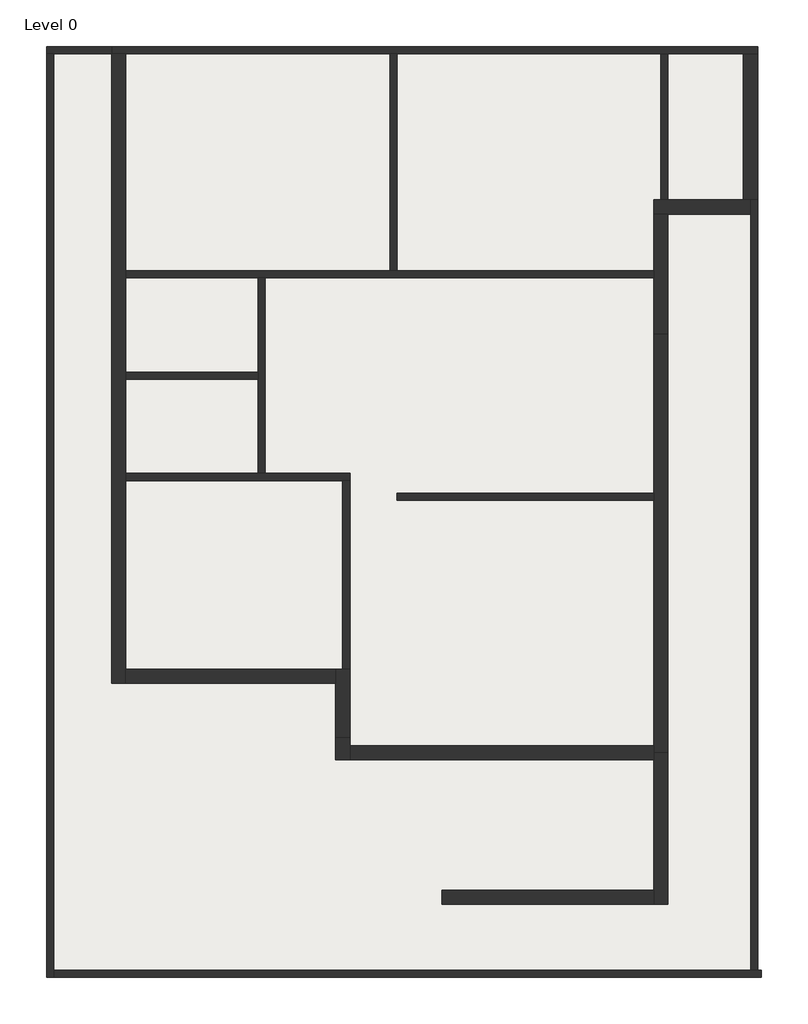
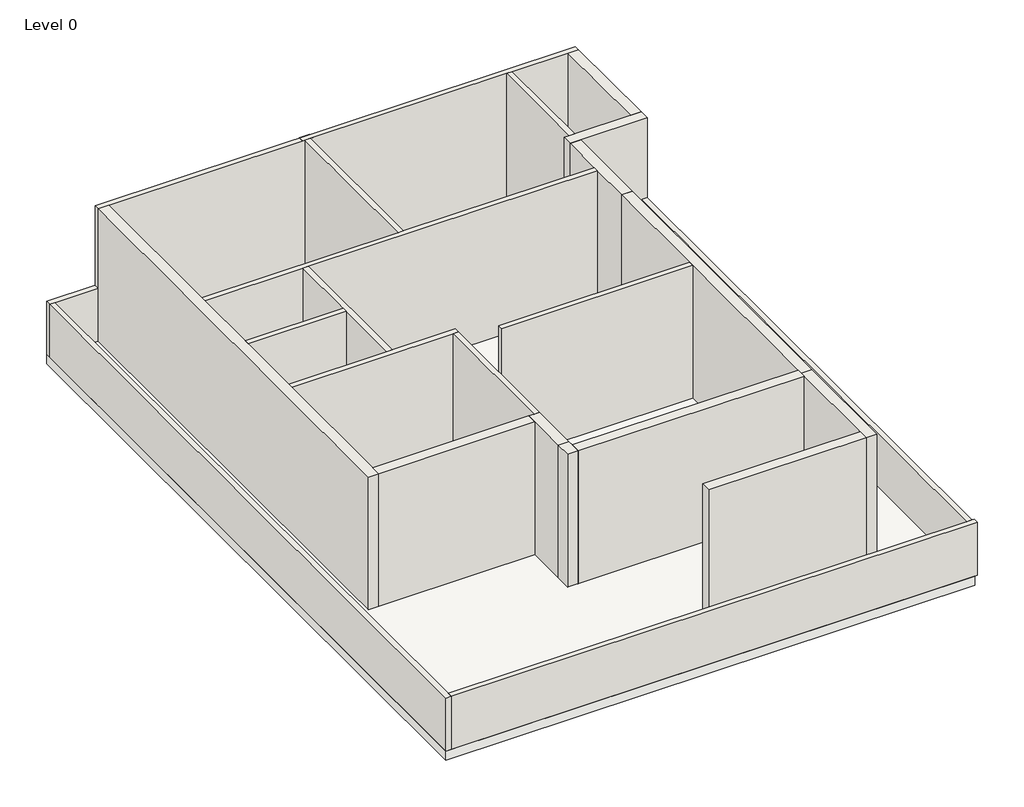
# One storey: 25 walls, 1 slab.
"""IFC4 building model written with IfcOpenShell, lengths in millimetres."""

from ifc_helpers import new_model, si_unit, frame, origin, origin_with_axes, place, context, project, spatial, polyline, outline, extrude, faceted_brep, element, save

model = new_model("IFC4")

# Units and contexts
model_context = context("Model", 3, world=origin())
ifc_project = project(units=[si_unit("LENGTHUNIT", "METRE", prefix="MILLI")], contexts=[model_context])

# Site, building, storey
site = spatial("IfcSite", under=ifc_project)
building = spatial("IfcBuilding", under=site)
storey = spatial("IfcBuildingStorey", under=building, Name="Level 0", Elevation=0.0)

# Slab
placement = place(None, origin())
element("IfcSlab", 1, at=placement, inside=storey, context=model_context, shape_type="SweptSolid", body=[
    extrude(outline(polyline([(5920.3326329, 7268.7468257), (5920.3326329, -7768.0531743), (-5573.1673671, -7768.0531743), (-5573.1673671, 7268.7468257), (5920.3326329, 7268.7468257)])), frame((0.0, 0.0, -211.0), z_axis=(0.0, 0.0, 1.0), x_axis=(1.0, 0.0, 0.0)), (0.0, 0.0, 1.0), 211.0),
])

# Walls
element("IfcWall", 2, ObjectType="INNER WALL-4.5\"", at=placement, inside=storey, context=model_context, shape_type="Brep", body=[
    faceted_brep([(-5573.1673671, 7154.4468257, 0.0), (-5458.8673671, 7154.4468257, 0.0), (-4519.0673671, 7154.4468257, 0.0), (-4519.0673671, 7154.4468257, 1219.2), (-5458.8673671, 7154.4468257, 1219.2), (-5573.1673671, 7154.4468257, 1219.2), (-5573.1673671, 7268.7468257, 0.0), (-5573.1673671, 7268.7468257, 1219.2), (-4519.0673671, 7268.7468257, 1219.2), (-4519.0673671, 7268.7468257, 0.0)], [[[0, 1, 2, 3, 4, 5]], [[6, 7, 8, 9]], [[2, 1, 0, 6, 9]], [[3, 2, 9, 8]], [[5, 4, 3, 8, 7]], [[0, 5, 7, 6]]]),
])
element("IfcWall", 3, ObjectType="INNER WALL-4.5\"", at=placement, inside=storey, context=model_context, shape_type="Brep", body=[
    faceted_brep([(-5573.1673671, 7154.4468257, 0.0), (-5573.1673671, -7768.0531743, 0.0), (-5573.1673671, -7768.0531743, 1219.2), (-5573.1673671, 7154.4468257, 1219.2), (-5458.8673671, 7154.4468257, 0.0), (-5458.8673671, 7154.4468257, 1219.2), (-5458.8673671, -7653.7531743, 1219.2), (-5458.8673671, -7768.0531743, 1219.2), (-5458.8673671, -7768.0531743, 0.0), (-5458.8673671, -7653.7531743, 0.0)], [[[0, 1, 2, 3]], [[4, 5, 6, 7, 8, 9]], [[1, 0, 4, 9, 8]], [[3, 2, 7, 6, 5]], [[0, 3, 5, 4]], [[2, 1, 8, 7]]]),
])
element("IfcWall", 4, ObjectType="INNER WALL-4.5\"", at=placement, inside=storey, context=model_context, shape_type="Brep", body=[
    faceted_brep([(5977.4826329, -7653.7531743, 0.0), (5920.3326329, -7653.7531743, 0.0), (5806.0326329, -7653.7531743, 0.0), (-5458.8673671, -7653.7531743, 0.0), (-5458.8673671, -7653.7531743, 1219.2), (5806.0326329, -7653.7531743, 1219.2), (5920.3326329, -7653.7531743, 1219.2), (5977.4826329, -7653.7531743, 1219.2), (5977.4826329, -7768.0531743, 0.0), (5977.4826329, -7768.0531743, 1219.2), (-5458.8673671, -7768.0531743, 1219.2), (-5458.8673671, -7768.0531743, 0.0)], [[[0, 1, 2, 3, 4, 5, 6, 7]], [[8, 9, 10, 11]], [[3, 2, 1, 0, 8, 11]], [[7, 6, 5, 4, 10, 9]], [[0, 7, 9, 8]], [[4, 3, 11, 10]]]),
])
element("IfcWall", 5, ObjectType="INNER WALL-4.5\"", at=placement, inside=storey, context=model_context, shape_type="Brep", body=[
    faceted_brep([(5806.0326329, 4792.2468257, 0.0), (5806.0326329, 4563.6468257, 0.0), (5806.0326329, -7653.7531743, 0.0), (5806.0326329, -7653.7531743, 1219.2), (5806.0326329, 4563.6468257, 1219.2), (5806.0326329, 4792.2468257, 1219.2), (5920.3326329, 4792.2468257, 0.0), (5920.3326329, 4792.2468257, 1219.2), (5920.3326329, 4563.6468257, 1219.2), (5920.3326329, -7653.7531743, 1219.2), (5920.3326329, -7653.7531743, 0.0)], [[[0, 1, 2, 3, 4, 5]], [[6, 7, 8, 9, 10]], [[2, 1, 0, 6, 10]], [[5, 4, 3, 9, 8, 7]], [[3, 2, 10, 9]], [[0, 5, 7, 6]]]),
])
element("IfcWall", 6, ObjectType="INNER WALL-4.5\"", at=placement, inside=storey, context=model_context, shape_type="Brep", body=[
    faceted_brep([(-4519.0673671, 7154.4468257, 0.0), (-4290.4673671, 7154.4468257, 0.0), (-23.2673671, 7154.4468257, 0.0), (91.0326329, 7154.4468257, 0.0), (4358.2326329, 7154.4468257, 0.0), (4472.5326329, 7154.4468257, 0.0), (5691.7326329, 7154.4468257, 0.0), (5920.3326329, 7154.4468257, 0.0), (5920.3326329, 7154.4468257, 3048.0), (5691.7326329, 7154.4468257, 3048.0), (4472.5326329, 7154.4468257, 3048.0), (4358.2326329, 7154.4468257, 3048.0), (91.0326329, 7154.4468257, 3048.0), (-23.2673671, 7154.4468257, 3048.0), (-4290.4673671, 7154.4468257, 3048.0), (-4519.0673671, 7154.4468257, 3048.0), (-4519.0673671, 7154.4468257, 1219.2), (-4519.0673671, 7268.7468257, 0.0), (-4519.0673671, 7268.7468257, 1219.2), (-4519.0673671, 7268.7468257, 3048.0), (5920.3326329, 7268.7468257, 3048.0), (5920.3326329, 7268.7468257, 0.0)], [[[0, 1, 2, 3, 4, 5, 6, 7, 8, 9, 10, 11, 12, 13, 14, 15, 16]], [[17, 18, 19, 20, 21]], [[7, 6, 5, 4, 3, 2, 1, 0, 17, 21]], [[15, 14, 13, 12, 11, 10, 9, 8, 20, 19]], [[0, 16, 15, 19, 18, 17]], [[8, 7, 21, 20]]]),
])
element("IfcWall", 7, ObjectType="INNER WALL-4.5\"", at=placement, inside=storey, context=model_context, shape_type="Brep", body=[
    faceted_brep([(148.1826329, 7268.7468257, 0.0), (-80.4173671, 7268.7468257, 0.0), (-80.4173671, 7268.7468257, 3048.0), (148.1826329, 7268.7468257, 3048.0), (148.1826329, 7154.4468257, 0.0), (148.1826329, 7154.4468257, 3048.0), (91.0326329, 7154.4468257, 3048.0), (-23.2673671, 7154.4468257, 3048.0), (-80.4173671, 7154.4468257, 3048.0), (-80.4173671, 7154.4468257, 0.0), (-23.2673671, 7154.4468257, 0.0), (91.0326329, 7154.4468257, 0.0)], [[[0, 1, 2, 3]], [[4, 5, 6, 7, 8, 9, 10, 11]], [[1, 0, 4, 11, 10, 9]], [[2, 1, 9, 8]], [[3, 2, 8, 7, 6, 5]], [[0, 3, 5, 4]]]),
])
element("IfcWall", 8, ObjectType="INNER WALL-4.5\"", at=placement, inside=storey, context=model_context, shape_type="SweptSolid", body=[
    extrude(outline(polyline([(-23.2673671, 3649.2468257), (-23.2673671, 7154.4468257), (91.0326329, 7154.4468257), (91.0326329, 3649.2468257), (-23.2673671, 3649.2468257)])), origin_with_axes(), (0.0, 0.0, 1.0), 3048.0),
])
element("IfcWall", 9, ObjectType="INNER WALL-4.5\"", at=placement, inside=storey, context=model_context, shape_type="Brep", body=[
    faceted_brep([(-4290.4673671, 3534.9468257, 0.0), (-2156.8673671, 3534.9468257, 0.0), (-2042.5673671, 3534.9468257, 0.0), (4243.9326329, 3534.9468257, 0.0), (4243.9326329, 3534.9468257, 3048.0), (-2042.5673671, 3534.9468257, 3048.0), (-2156.8673671, 3534.9468257, 3048.0), (-4290.4673671, 3534.9468257, 3048.0), (-4290.4673671, 3649.2468257, 0.0), (-4290.4673671, 3649.2468257, 3048.0), (-23.2673671, 3649.2468257, 3048.0), (91.0326329, 3649.2468257, 3048.0), (4243.9326329, 3649.2468257, 3048.0), (4243.9326329, 3649.2468257, 0.0), (91.0326329, 3649.2468257, 0.0), (-23.2673671, 3649.2468257, 0.0)], [[[0, 1, 2, 3, 4, 5, 6, 7]], [[8, 9, 10, 11, 12, 13, 14, 15]], [[3, 2, 1, 0, 8, 15, 14, 13]], [[7, 6, 5, 4, 12, 11, 10, 9]], [[0, 7, 9, 8]], [[4, 3, 13, 12]]]),
])
element("IfcWall", 10, ObjectType="INNER WALL-4.5\"", at=placement, inside=storey, context=model_context, shape_type="Brep", body=[
    faceted_brep([(-2156.8673671, 3534.9468257, 0.0), (-2156.8673671, 2010.9468257, 0.0), (-2156.8673671, 1896.6468257, 0.0), (-2156.8673671, 372.6468257, 0.0), (-2156.8673671, 372.6468257, 3048.0), (-2156.8673671, 1896.6468257, 3048.0), (-2156.8673671, 2010.9468257, 3048.0), (-2156.8673671, 3534.9468257, 3048.0), (-2042.5673671, 3534.9468257, 0.0), (-2042.5673671, 3534.9468257, 3048.0), (-2042.5673671, 372.6468257, 3048.0), (-2042.5673671, 372.6468257, 0.0)], [[[0, 1, 2, 3, 4, 5, 6, 7]], [[8, 9, 10, 11]], [[3, 2, 1, 0, 8, 11]], [[7, 6, 5, 4, 10, 9]], [[0, 7, 9, 8]], [[4, 3, 11, 10]]]),
])
element("IfcWall", 11, ObjectType="INNER WALL-4.5\"", at=placement, inside=storey, context=model_context, shape_type="Brep", body=[
    faceted_brep([(-4290.4673671, 258.3468257, 0.0), (-785.2673671, 258.3468257, 0.0), (-670.9673671, 258.3468257, 0.0), (-670.9673671, 258.3468257, 3048.0), (-785.2673671, 258.3468257, 3048.0), (-4290.4673671, 258.3468257, 3048.0), (-4290.4673671, 372.6468257, 0.0), (-4290.4673671, 372.6468257, 3048.0), (-2156.8673671, 372.6468257, 3048.0), (-2042.5673671, 372.6468257, 3048.0), (-670.9673671, 372.6468257, 3048.0), (-670.9673671, 372.6468257, 0.0), (-2042.5673671, 372.6468257, 0.0), (-2156.8673671, 372.6468257, 0.0)], [[[0, 1, 2, 3, 4, 5]], [[6, 7, 8, 9, 10, 11, 12, 13]], [[2, 1, 0, 6, 13, 12, 11]], [[5, 4, 3, 10, 9, 8, 7]], [[0, 5, 7, 6]], [[3, 2, 11, 10]]]),
])
element("IfcWall", 12, ObjectType="INNER WALL-4.5\"", at=placement, inside=storey, context=model_context, shape_type="SweptSolid", body=[
    extrude(outline(polyline([(-2156.8673671, 1896.6468257), (-4290.4673671, 1896.6468257), (-4290.4673671, 2010.9468257), (-2156.8673671, 2010.9468257), (-2156.8673671, 1896.6468257)])), origin_with_axes(), (0.0, 0.0, 1.0), 3048.0),
])
element("IfcWall", 13, ObjectType="INNER WALL-4.5\"", at=placement, inside=storey, context=model_context, shape_type="SweptSolid", body=[
    extrude(outline(polyline([(-785.2673671, -2789.6531743), (-785.2673671, 258.3468257), (-670.9673671, 258.3468257), (-670.9673671, -2789.6531743), (-785.2673671, -2789.6531743)])), origin_with_axes(), (0.0, 0.0, 1.0), 3048.0),
])
element("IfcWall", 14, ObjectType="INNER WALL-4.5\"", at=placement, inside=storey, context=model_context, shape_type="SweptSolid", body=[
    extrude(outline(polyline([(4243.9326329, -59.1531743), (91.0326329, -59.1531743), (91.0326329, 55.1468257), (4243.9326329, 55.1468257), (4243.9326329, -59.1531743)])), origin_with_axes(), (0.0, 0.0, 1.0), 3048.0),
])
element("IfcWall", 15, ObjectType="INNER WALL-4.5\"", at=placement, inside=storey, context=model_context, shape_type="SweptSolid", body=[
    extrude(outline(polyline([(4358.2326329, 4792.2468257), (4358.2326329, 7154.4468257), (4472.5326329, 7154.4468257), (4472.5326329, 4792.2468257), (4358.2326329, 4792.2468257)])), origin_with_axes(), (0.0, 0.0, 1.0), 3048.0),
])
element("IfcWall", 16, ObjectType="OUTER WALL-9\"", at=placement, inside=storey, context=model_context, shape_type="Brep", body=[
    faceted_brep([(-4519.0673671, 7154.4468257, 3048.0), (-4519.0673671, 7154.4468257, 0.0), (-4519.0673671, -3018.2531743, 0.0), (-4519.0673671, -3018.2531743, 3048.0), (-4290.4673671, 7154.4468257, 0.0), (-4290.4673671, 7154.4468257, 3048.0), (-4290.4673671, 3649.2468257, 3048.0), (-4290.4673671, 3534.9468257, 3048.0), (-4290.4673671, 2010.9468257, 3048.0), (-4290.4673671, 1896.6468257, 3048.0), (-4290.4673671, 372.6468257, 3048.0), (-4290.4673671, 258.3468257, 3048.0), (-4290.4673671, -2789.6531743, 3048.0), (-4290.4673671, -3018.2531743, 3048.0), (-4290.4673671, -3018.2531743, 0.0), (-4290.4673671, -2789.6531743, 0.0), (-4290.4673671, 258.3468257, 0.0), (-4290.4673671, 372.6468257, 0.0), (-4290.4673671, 1896.6468257, 0.0), (-4290.4673671, 2010.9468257, 0.0), (-4290.4673671, 3534.9468257, 0.0), (-4290.4673671, 3649.2468257, 0.0)], [[[0, 1, 2, 3]], [[4, 5, 6, 7, 8, 9, 10, 11, 12, 13, 14, 15, 16, 17, 18, 19, 20, 21]], [[2, 1, 4, 21, 20, 19, 18, 17, 16, 15, 14]], [[0, 3, 13, 12, 11, 10, 9, 8, 7, 6, 5]], [[3, 2, 14, 13]], [[0, 5, 4, 1]]]),
])
element("IfcWall", 17, ObjectType="OUTER WALL-9\"", at=placement, inside=storey, context=model_context, shape_type="SweptSolid", body=[
    extrude(outline(polyline([(-899.5673671, -3018.2531743), (-4290.4673671, -3018.2531743), (-4290.4673671, -2789.6531743), (-899.5673671, -2789.6531743), (-899.5673671, -3018.2531743)])), origin_with_axes(), (0.0, 0.0, 1.0), 3048.0),
])
element("IfcWall", 18, ObjectType="OUTER WALL-9\"", at=placement, inside=storey, context=model_context, shape_type="Brep", body=[
    faceted_brep([(-899.5673671, -3896.2596162, 0.0), (-899.5673671, -4250.1531743, 0.0), (-899.5673671, -4250.1531743, 3048.0), (-899.5673671, -3896.2596162, 3048.0), (-670.9673671, -3896.2596162, 0.0), (-670.9673671, -3896.2596162, 3048.0), (-670.9673671, -4021.5531743, 3048.0), (-670.9673671, -4250.1531743, 3048.0), (-670.9673671, -4250.1531743, 0.0), (-670.9673671, -4021.5531743, 0.0)], [[[0, 1, 2, 3]], [[4, 5, 6, 7, 8, 9]], [[1, 0, 4, 9, 8]], [[3, 2, 7, 6, 5]], [[0, 3, 5, 4]], [[2, 1, 8, 7]]]),
])
element("IfcWall", 19, ObjectType="OUTER WALL-9\"", at=placement, inside=storey, context=model_context, shape_type="Brep", body=[
    faceted_brep([(-670.9673671, -3896.2596162, 0.0), (-670.9673671, -2789.6531743, 0.0), (-670.9673671, -2789.6531743, 3048.0), (-670.9673671, -3896.2596162, 3048.0), (-899.5673671, -3896.2596162, 0.0), (-899.5673671, -3896.2596162, 3048.0), (-899.5673671, -3018.2531743, 3048.0), (-899.5673671, -2789.6531743, 3048.0), (-899.5673671, -2789.6531743, 0.0), (-899.5673671, -3018.2531743, 0.0), (-785.2673671, -2789.6531743, 0.0), (-785.2673671, -2789.6531743, 3048.0)], [[[0, 1, 2, 3]], [[4, 5, 6, 7, 8, 9]], [[1, 0, 4, 9, 8, 10]], [[3, 2, 11, 7, 6, 5]], [[0, 3, 5, 4]], [[2, 1, 10, 8, 7, 11]]]),
])
element("IfcWall", 20, ObjectType="OUTER WALL-9\"", at=placement, inside=storey, context=model_context, shape_type="Brep", body=[
    faceted_brep([(4472.5326329, -6586.9531743, 0.0), (4472.5326329, -4135.8531743, 0.0), (4472.5326329, -4135.8531743, 3048.0), (4472.5326329, -6586.9531743, 3048.0), (4243.9326329, -6586.9531743, 0.0), (4243.9326329, -6586.9531743, 3048.0), (4243.9326329, -6358.3531743, 3048.0), (4243.9326329, -4250.1531743, 3048.0), (4243.9326329, -4135.8531743, 3048.0), (4243.9326329, -4135.8531743, 0.0), (4243.9326329, -4250.1531743, 0.0), (4243.9326329, -6358.3531743, 0.0)], [[[0, 1, 2, 3]], [[4, 5, 6, 7, 8, 9, 10, 11]], [[1, 0, 4, 11, 10, 9]], [[2, 1, 9, 8]], [[3, 2, 8, 7, 6, 5]], [[0, 3, 5, 4]]]),
])
element("IfcWall", 21, ObjectType="OUTER WALL-9\"", at=placement, inside=storey, context=model_context, shape_type="SweptSolid", body=[
    extrude(outline(polyline([(4243.9326329, -6586.9531743), (818.3954901, -6586.9531743), (818.3954901, -6358.3531743), (4243.9326329, -6358.3531743), (4243.9326329, -6586.9531743)])), origin_with_axes(), (0.0, 0.0, 1.0), 3048.0),
])
element("IfcWall", 22, ObjectType="OUTER WALL-9\"", at=placement, inside=storey, context=model_context, shape_type="Brep", body=[
    faceted_brep([(4472.5326329, -4135.8531743, 0.0), (4472.5326329, 2620.5468257, 0.0), (4472.5326329, 2620.5468257, 3048.0), (4472.5326329, -4135.8531743, 3048.0), (4243.9326329, -4135.8531743, 0.0), (4243.9326329, -4135.8531743, 3048.0), (4243.9326329, -4021.5531743, 3048.0), (4243.9326329, -59.1531743, 3048.0), (4243.9326329, 55.1468257, 3048.0), (4243.9326329, 2620.5468257, 3048.0), (4243.9326329, 2620.5468257, 0.0), (4243.9326329, 55.1468257, 0.0), (4243.9326329, -59.1531743, 0.0), (4243.9326329, -4021.5531743, 0.0)], [[[0, 1, 2, 3]], [[4, 5, 6, 7, 8, 9, 10, 11, 12, 13]], [[1, 0, 4, 13, 12, 11, 10]], [[2, 1, 10, 9]], [[3, 2, 9, 8, 7, 6, 5]], [[0, 3, 5, 4]]]),
])
element("IfcWall", 23, ObjectType="OUTER WALL-9\"", at=placement, inside=storey, context=model_context, shape_type="Brep", body=[
    faceted_brep([(-670.9673671, -4250.1531743, 0.0), (4243.9326329, -4250.1531743, 0.0), (4243.9326329, -4250.1531743, 3048.0), (-670.9673671, -4250.1531743, 3048.0), (-670.9673671, -4021.5531743, 0.0), (-670.9673671, -4021.5531743, 3048.0), (4243.9326329, -4021.5531743, 3048.0), (4243.9326329, -4021.5531743, 0.0), (4243.9326329, -4135.8531743, 0.0), (4243.9326329, -4135.8531743, 3048.0)], [[[0, 1, 2, 3]], [[4, 5, 6, 7]], [[1, 0, 4, 7, 8]], [[3, 2, 9, 6, 5]], [[0, 3, 5, 4]], [[2, 1, 8, 7, 6, 9]]]),
])
element("IfcWall", 24, ObjectType="OUTER WALL-9\"", at=placement, inside=storey, context=model_context, shape_type="Brep", body=[
    faceted_brep([(4243.9326329, 4563.6468257, 0.0), (4472.5326329, 4563.6468257, 0.0), (5806.0326329, 4563.6468257, 0.0), (5806.0326329, 4563.6468257, 1219.2), (5920.3326329, 4563.6468257, 1219.2), (5920.3326329, 4563.6468257, 3048.0), (4472.5326329, 4563.6468257, 3048.0), (4243.9326329, 4563.6468257, 3048.0), (4243.9326329, 4792.2468257, 0.0), (4243.9326329, 4792.2468257, 3048.0), (4358.2326329, 4792.2468257, 3048.0), (4472.5326329, 4792.2468257, 3048.0), (5691.7326329, 4792.2468257, 3048.0), (5920.3326329, 4792.2468257, 3048.0), (5920.3326329, 4792.2468257, 1219.2), (5806.0326329, 4792.2468257, 1219.2), (5806.0326329, 4792.2468257, 0.0), (5691.7326329, 4792.2468257, 0.0), (4472.5326329, 4792.2468257, 0.0), (4358.2326329, 4792.2468257, 0.0)], [[[0, 1, 2, 3, 4, 5, 6, 7]], [[8, 9, 10, 11, 12, 13, 14, 15, 16, 17, 18, 19]], [[2, 1, 0, 8, 19, 18, 17, 16]], [[7, 6, 5, 13, 12, 11, 10, 9]], [[14, 4, 3, 15]], [[3, 2, 16, 15]], [[5, 4, 14, 13]], [[0, 7, 9, 8]]]),
])
element("IfcWall", 25, ObjectType="OUTER WALL-9\"", at=placement, inside=storey, context=model_context, shape_type="Brep", body=[
    faceted_brep([(5691.7326329, 7154.4468257, 0.0), (5691.7326329, 4792.2468257, 0.0), (5691.7326329, 4792.2468257, 3048.0), (5691.7326329, 7154.4468257, 3048.0), (5920.3326329, 7154.4468257, 0.0), (5920.3326329, 7154.4468257, 3048.0), (5920.3326329, 4792.2468257, 3048.0), (5920.3326329, 4792.2468257, 1219.2), (5920.3326329, 4792.2468257, 0.0), (5806.0326329, 4792.2468257, 0.0)], [[[0, 1, 2, 3]], [[4, 5, 6, 7, 8]], [[1, 0, 4, 8, 9]], [[3, 2, 6, 5]], [[0, 3, 5, 4]], [[2, 1, 9, 8, 7, 6]]]),
])
element("IfcWall", 26, ObjectType="OUTER WALL-9\"", at=placement, inside=storey, context=model_context, shape_type="Brep", body=[
    faceted_brep([(4243.9326329, 4563.6468257, 0.0), (4243.9326329, 3649.2468257, 0.0), (4243.9326329, 3534.9468257, 0.0), (4243.9326329, 2620.5468257, 0.0), (4243.9326329, 2620.5468257, 3048.0), (4243.9326329, 3534.9468257, 3048.0), (4243.9326329, 3649.2468257, 3048.0), (4243.9326329, 4563.6468257, 3048.0), (4472.5326329, 4563.6468257, 0.0), (4472.5326329, 4563.6468257, 3048.0), (4472.5326329, 2620.5468257, 3048.0), (4472.5326329, 2620.5468257, 0.0)], [[[0, 1, 2, 3, 4, 5, 6, 7]], [[8, 9, 10, 11]], [[3, 2, 1, 0, 8, 11]], [[4, 3, 11, 10]], [[7, 6, 5, 4, 10, 9]], [[0, 7, 9, 8]]]),
])

save(model, "model.ifc")

# Revit data of these elements
# Type
#   Function = 0
#   Layers, outside or top first: 0.692257 ft "Concrete, Cast-in-Place - C15" (function 1); 0.0 ft "Metal Deck" (function 200)
# Type "INNER WALL-4.5\""
#   Layers, outside or top first: 0.375 ft "Concrete, Cast In Situ" (function 1)
# Type "OUTER WALL-9\""
#   Layers, outside or top first: 0.75 ft "Concrete, Cast In Situ" (function 1)
# Element 1 (IfcSlab)
#   Height Offset From Level = 0.0 ft
#   Phase Created = New Construction
#   Materials on its faces: "Metal Deck", "Concrete, Cast-in-Place - C15"
# Elements 2, 3, 4, 5 (IfcWall, "INNER WALL-4.5\"")
#   Top Offset = 0.0 ft
#   Base Offset = 0.0 ft
#   Unconnected Height = 4.0 ft
#   wall height = 4.0 ft
#   Phase Created = New Construction
#   Base Constraint = Level 0
#   Materials on its faces: "Concrete, Cast In Situ"
# Elements 6, 7, 8, 9, 10, 11, 12, 13, 14, 15 (IfcWall, "INNER WALL-4.5\"")
#   Top Offset = 0.0 ft
#   Base Offset = 0.0 ft
#   Unconnected Height = 10.0 ft
#   wall height = 10.0 ft
#   Phase Created = New Construction
#   Base Constraint = Level 0
#   Materials on its faces: "Concrete, Cast In Situ"
# Elements 16, 17, 18, 19, 20, 21, 22, 23, 24, 25, 26 (IfcWall, "OUTER WALL-9\"")
#   Top Offset = 0.0 ft
#   Base Offset = 0.0 ft
#   Unconnected Height = 10.0 ft
#   wall height = 10.0 ft
#   Phase Created = New Construction
#   Base Constraint = Level 0
#   Materials on its faces: "Concrete, Cast In Situ"
# Materials
#   "Concrete, Cast-in-Place - C15": class "Concrete", colour RGB 192 192 192, transparency 0, Description = "Concrete 15 MPa", Cost = 0
#   "Metal Deck": class "Metal", colour RGB 247 247 247, transparency 0, Description = "Steel, mill finish", Cost = 0
#   "Concrete, Cast In Situ": class "Concrete", colour RGB 192 192 192, transparency 0, Description = "physical material", Cost = 0
# Room, not placed, phase "New Construction", upper offset 0.0 ft, lower offset 0.0 ft
#   Number = "1"
#   Name = "Room"
# Room, not placed, phase "New Construction", upper offset 0.0 ft, lower offset 0.0 ft
#   Number = "2"
#   Name = "Room"
